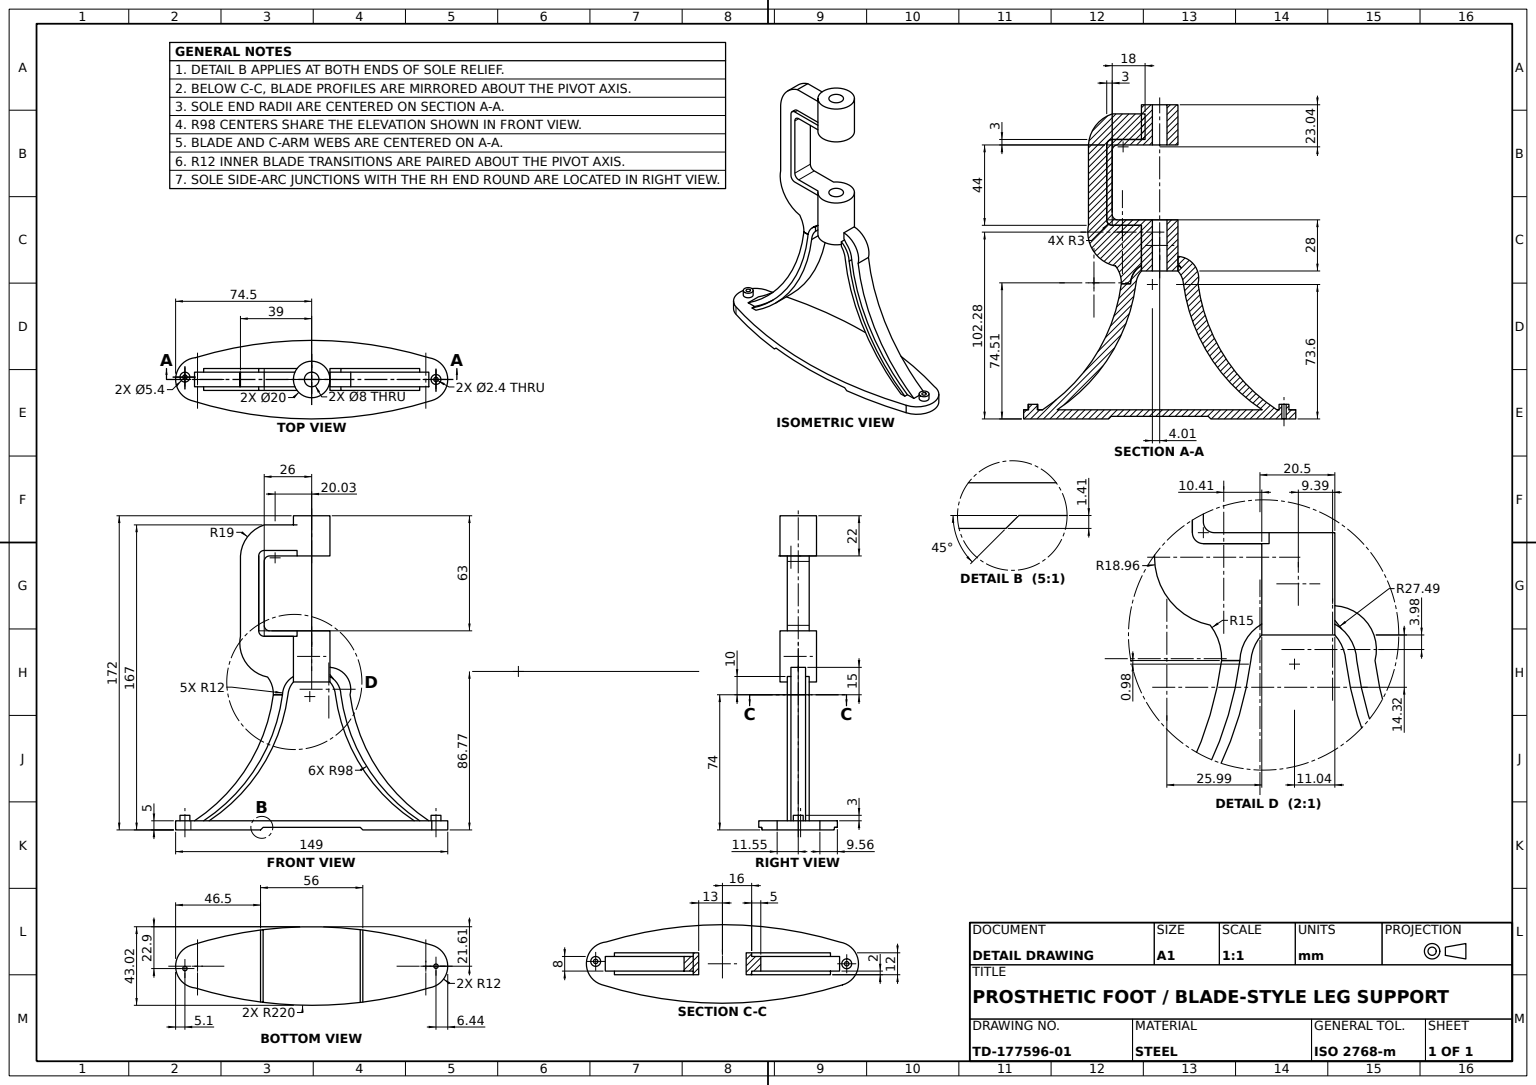
SolidWorks part; units mm, degrees
material "Plain Carbon Steel"
ref_plane "Front Plane" through (0, 0, 0) normal (0, 0, 1) x (1, 0, 0)
ref_plane "Top Plane" through (0, 0, 0) normal (0, 1, 0) x (1, 0, 0)
ref_plane "Right Plane" through (0, 0, 0) normal (1, 0, 0) x (0, 0, -1)
sketch "Base Plate Sketch" plane through (0, 0, 0) normal (0, 1, 0) x (1, 0, 0)
  arc A0 (-63.6181, 11.9478) -> (-66.0643, -11.4584) centre (-62.5, 0) ccw
  arc A1 (65.7488, -11.5518) -> (64.3661, 11.854) centre (62.5, 0) ccw
  arc A2 (-63.6181, 11.9478) -> (64.3661, 11.854) centre (0.2198, -198.5866) cw
  arc A3 (65.7488, -11.5518) -> (-66.1462, -11.4327) centre (-0.009, 198.3908) cw
  dimension "D1" = 24
  dimension "D2" = 24
  dimension "D3" = 62.5
  dimension "D6" = 220
  dimension "D7" = 220
  dimension "D8" = 198.3908
  dimension "D4" = 62.5
  dimension "D5" = 125
  dimension "D9" = 1.3827
  dimension "D10" = 3.2488
  dimension "D11" = 65.5291
extrude "Base Plate" add sketch "Base Plate Sketch" along normal blind 5 contours A3 A1 A2 A0
ref_plane "Plane1" through (0, 0, 0) normal (0, 0, 1) x (1, 0, 0)
ref_plane "Plane2" through (0, 172, 0) normal (0, 1, 0) x (1, 0, 0)
sketch "Upper Pivot Boss Sketch" plane through (0, 172, 0) normal (0, 1, 0) x (1, 0, 0)
  circle A0 centre (0, 0) radius 10
  dimension "D1" = 20
extrude "Upper Pivot Boss" add sketch "Upper Pivot Boss Sketch" against normal blind 22 separate body
ref_plane "Plane3" through (0, 109, 0) normal (0, 1, 0) x (1, 0, 0)
sketch "Lower Pivot Boss Sketch" plane through (0, 109, 0) normal (0, 1, 0) x (1, 0, 0)
  circle A0 centre (0, 0) radius 10
  dimension "D1" = 20
extrude "Lower Pivot Boss" add sketch "Lower Pivot Boss Sketch" against normal blind 28 separate body
sketch "Support Legs Sketch" plane through (0, 0, 0) normal (0, 0, 1) x (1, 0, 0)
  line L2 (-56.1462, 5) -> (-59.1462, 5)
  line L3 (64.3661, 5) -> (-63.6181, 5) construction
  line L8 (65.7488, 5) -> (-66.1462, 5) construction
  line L9 (56.1462, 5) -> (59.1462, 5)
  line L12 (-10, 81) -> (-10, 84)
  line L13 (-10, 109) -> (-10, 81) construction
  line L15 (10, 81) -> (10, 84)
  arc A0 (-13, 74) -> (-56.1462, 5) centre (-110.1647, 86.7679) cw
  arc A1 (-16, 74) -> (-59.1462, 5) centre (-113.1647, 86.7679) cw
  arc A2 (13, 74) -> (56.1462, 5) centre (110.1647, 86.7679) ccw
  arc A3 (16, 74) -> (59.1462, 5) centre (113.1647, 86.7679) ccw
  arc A4 (-13, 74) -> (-10, 81) centre (-1.0403, 73.0173) cw
  arc A5 (-16, 74) -> (-10, 84) centre (-4.0065, 73.6039) cw
  arc A6 (13, 74) -> (10, 81) centre (1.0403, 73.0173) ccw
  arc A7 (16, 74) -> (10, 84) centre (4.0065, 73.6039) ccw
  dimension "D3" = 98
  dimension "D4" = 20
  dimension "D5" = 98
  dimension "D6" = 13
  dimension "D7" = 3
  dimension "D8" = 12
  dimension "D10" = 12
  dimension "D2" = 74
  dimension "D9" = 3
  dimension "D11" = 86.7679
extrude "Support Legs" add sketch "Support Legs Sketch" along normal mid plane 12
sketch "C-Arm Sketch" plane through (0, 0, 0) normal (0, 0, 1) x (1, 0, 0)
  line L1 (-10, 153) -> (-26, 153)
  line L2 (-29, 150) -> (-29, 109)
  line L3 (-26, 106) -> (-10, 106)
  line L4 (-10, 109) -> (-10, 81) construction
  line L6 (23.6624, 109) -> (-23.6624, 109) construction
  line L7 (-10, 109) -> (-23, 109)
  line L8 (-26, 112) -> (-26, 147)
  line L9 (-23, 150) -> (-10, 150)
  line L10 (-10, 109) -> (-7.951, 109)
  line L11 (-7.951, 109) -> (-7.951, 106)
  line L12 (-7.951, 106) -> (-10, 106)
  line L13 (-10, 153) -> (-7.951, 153)
  line L14 (-7.951, 153) -> (-7.951, 150)
  line L15 (-10, 150) -> (10, 150) construction
  line L16 (-7.951, 150) -> (-10, 150)
  arc A0 (-23, 109) -> (-26, 112) centre (-23, 112) cw
  arc A1 (-29, 109) -> (-26, 106) centre (-26, 109) ccw
  arc A2 (-26, 147) -> (-23, 150) centre (-23, 147) cw
  arc A3 (-26, 153) -> (-29, 150) centre (-26, 150) ccw
  point P15 (-26, 109)
  dimension "D1" = 3
  dimension "D2" = 16
  dimension "D3" = 3
  dimension "D4" = 3
  dimension "D5" = 3
  dimension "D6" = 2.049
extrude "C-Arm" add sketch "C-Arm Sketch" along normal mid plane 12
sketch "Leg Ribs Sketch" plane through (0, 0, 0) normal (0, 0, 1) x (1, 0, 0)
  line L0 (-59.1462, 5) -> (-64.1462, 5)
  line L1 (59.1462, 5) -> (64.1462, 5)
  line L2 (74.5, 5) -> (64.3661, 5) construction
  line L4 (59.1462, 5) -> (64.1462, 5)
  line L5 (-16, 74) -> (-21, 74)
  line L7 (10, 81) -> (10, 89)
  line L8 (10, 81) -> (10, 109) construction
  arc A0 (-21, 74) -> (-64.1462, 5) centre (-118.1647, 86.7679) cw
  arc A1 (21, 74) -> (64.1462, 5) centre (118.1647, 86.7679) ccw
  arc A2 (10, 89) -> (21, 74) centre (9.3851, 77.0158) cw
  arc A3 (-16, 74) -> (-59.1462, 5) centre (-113.1647, 86.7679) cw
  arc A4 (16, 74) -> (10, 85) centre (-10.4993, 66.6822) ccw
  arc A5 (16, 74) -> (59.1462, 5) centre (113.1647, 86.7679) ccw
  dimension "D3" = 8
  dimension "D4" = 98
  dimension "D5" = 12
  dimension "D6" = 27.4911
  dimension "D1" = 5
  dimension "D2" = 5
  dimension "D7" = 11
  dimension "D8" = 49.1462
  dimension "D9" = 26
extrude "Leg Ribs" add sketch "Leg Ribs Sketch" along normal mid plane 8 contours A3 L5 A0 L0 | A4 A5 L1 A1 A2 L7
sketch "C-Arm Rib Sketch" plane through (0, 0, 0) normal (0, 0, 1) x (1, 0, 0)
  line L0 (-16, 74) -> (-21, 74) construction
  line L1 (-39, 150) -> (-39, 106)
  line L2 (-10, 106) -> (-10, 81) construction
  line L3 (-8, 153) -> (-8, 167)
  line L4 (-8, 167) -> (-26, 167)
  line L6 (-26, 106) -> (-8, 106) construction
  line L7 (-29, 150) -> (-29, 109) construction
  line L8 (-8, 153) -> (-26, 153) construction
  line L9 (-16, 74) -> (-21, 74)
  line L10 (-10, 106) -> (-10, 84)
  line L11 (-26, 106) -> (-10, 106)
  line L12 (-29, 150) -> (-29, 109)
  line L13 (-8, 153) -> (-26, 153)
  arc A0 (-39, 150) -> (-26, 167) centre (-20.0283, 148.9628) cw
  arc A1 (-24.13, 83.6932) -> (-21, 74) centre (-35.9913, 74.5111) cw
  arc A2 (-24.13, 83.6932) -> (-39, 106) centre (-20.4116, 102.2816) cw
  arc A3 (-10, 84) -> (-16, 74) centre (-4.0065, 73.6039) ccw construction
  arc A4 (-26, 153) -> (-29, 150) centre (-26, 150) ccw construction
  arc A5 (-10, 84) -> (-16, 74) centre (-4.0065, 73.6039) ccw
  arc A6 (-26, 153) -> (-29, 150) centre (-26, 150) ccw
  arc A7 (-29, 109) -> (-26, 106) centre (-26, 109) ccw construction
  arc A8 (-29, 109) -> (-26, 106) centre (-26, 109) ccw
  dimension "D3" = 18
  dimension "D5" = 19
  dimension "D8" = 15
  dimension "D9" = 74.5111
  dimension "D10" = 18.9567
  dimension "D11" = 102.2816
  dimension "D1" = 44
  dimension "D2" = 39
  dimension "D4" = 167
extrude "C-Arm Rib" add sketch "C-Arm Rib Sketch" along normal mid plane 8 separate body
sketch "Pivot Bore Sketch" plane through (0, 172, 0) normal (0, 1, 0) x (1, 0, 0)
  circle A0 centre (0, 0) radius 4
  dimension "D1" = 8
extrude "Pivot Bore" cut sketch "Pivot Bore Sketch" against normal blind 128
sketch "Base Screw Bosses Sketch" plane through (0, 5, 0) normal (0, 1, 0) x (1, 0, 0)
  line L0 (-64.1462, -4) -> (-64.1462, 4) construction
  line L1 (-59.1462, -4) -> (-64.1462, -4) construction
  circle A0 centre (68.0595, 0) radius 2.6977
  circle A1 centre (-69.4038, 1.29) radius 2.7
  dimension "D1" = 5.4
  dimension "D2" = 5.3955
  dimension "D3" = 132.2057
  dimension "D4" = 5.2576
  dimension "D5" = 4
  dimension "D6" = 5.29
extrude "Base Screw Bosses" add sketch "Base Screw Bosses Sketch" along normal blind 3
sketch "Base Screw Holes Sketch" plane through (0, 8, 0) normal (0, 1, 0) x (1, 0, 0)
  circle A0 centre (68.0595, 0) radius 1.2
  circle A1 centre (-69.4038, 1.29) radius 1.2
  dimension "D1" = 2.4
extrude "Base Screw Holes" cut sketch "Base Screw Holes Sketch" against normal blind 33
ref_plane "Plane4" through (0, 0, 22) normal (0, 0, 1) x (1, 0, 0)
sketch "Profile Trim Sketch" plane through (0, 0, 22) normal (0, 0, 1) x (1, 0, 0)
  line L0 (0, 0) -> (28, 0)
  line L1 (-66.1462, 0) -> (65.7488, 0) construction
  line L2 (28, 0) -> (26.5858, 1.4142)
  line L3 (0, 0) -> (-28, 0)
  line L4 (-28, 0) -> (-26.5858, 1.4142)
  line L5 (-26.5858, 1.4142) -> (26.5858, 1.4142)
  dimension "D1" = 1.4142
  dimension "D2" = 28
  dimension "D3" = 1.4142
extrude "Profile Trim Cut" cut sketch "Profile Trim Sketch" against normal blind 59
